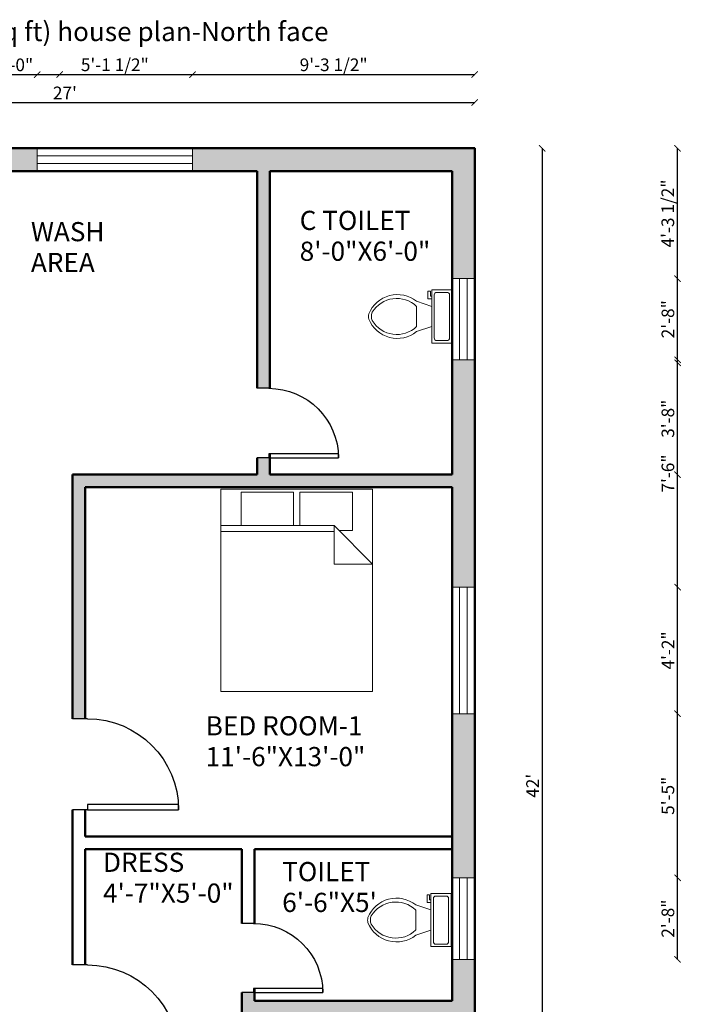
# Model space of a CAD drawing. Units: inches. Extents: x 1799 to 2247, y 1296 to 1881.
# Tile 4 of 4: x 1983 to 2247, y 1492 to 1881. Entities that reach past the tile are written whole.
import ezdxf

# ---------------------------------------------------------------- set-up
doc = ezdxf.new("R2010")
doc.units = ezdxf.units.IN
for name, color, linetype, lineweight in [('A-ANNO-DIMS', 2, 'Continuous', 18), ('A-ANNO-TEXT', 7, 'Continuous', 35), ('A-AREA-IDEN', 7, 'Continuous', 25), ('A-DOOR', 3, 'Continuous', 25), ('A-FLOR-FIXT', 9, 'Continuous', 18), ('A-FURN', 8, 'Continuous', 18), ('A-WALL', 7, 'Continuous', 50), ('window', 4, 'Continuous', 18)]:
    doc.layers.add(name, color=color, linetype=linetype, lineweight=lineweight)
doc.layers.add('A-WALL-PATT', color=18, linetype='Continuous', lineweight=13, true_color=0x000000)
doc.styles.get("Standard").update_dxf_attribs({"font": 'arial.ttf'})
doc.dimstyles.new('ISO-25', dxfattribs={"dimtxt": 5, "dimasz": 2.5, "dimexe": 1.25, "dimexo": 0.625, "dimtad": 1, "dimdec": 0, "dimlunit": 4, "dimtxsty": 'Standard', "dimblk": 'ARCHTICK', "dimcen": 2.5, "dimse1": 1, "dimse2": 1, "dimclrd": 1, "dimadec": 0, "dimazin": 0, "dimtfac": 1, "dimtdec": 0, "dimtmove": 0, "dimatfit": 3, "dimfxl": 1, "dimarcsym": 0})

# ---------------------------------------------------------------- blocks, each defined once
blk = doc.blocks.new('*U11')
for p, q in [((9.5, -6), (9.5, -2)), ((-10, -8.5), (-8, -8.5)), ((-10, -9.5), (-10, -8.5)), ((-7, -9.5), (-10, -9.5)), ((-8, -8.5), (-8, -8)), ((-7, -8), (-7, -9.5)), ((-4, -8), (-6, -14)), ((4, -8), (6, -14)), ((4, -14), (-4, -14))]:
    blk.add_line(p, q)
blk.add_lwpolyline([(10.5, -8), (10.5, 0), (-10.5, 0), (-10.5, -8)], close=True)
for points in [[(-9.5, -2), (-9.5, -6)], [(8.5, -1), (-8.5, -1)], [(-8.5, -7), (8.5, -7)]]:
    blk.add_lwpolyline(points)
for centre, radius, start, end in [((-8.62, -1.88), 0.884, 81.8699, 188.1301), ((8.62, -1.88), 0.884, 351.8699, 98.1301), ((-8.62, -6.12), 0.884, 171.8699, 278.1301), ((8.62, -6.12), 0.884, 261.8699, 8.1301), ((3.52, -21.58), 12.17, 141.4691, 247.9714), ((4.2, -21.82), 11.33, 136.3677, 238.9468), ((-3.52, -21.58), 12.17, 292.0284, 38.5307), ((-4.2, -21.82), 11.33, 301.053, 43.6321), ((0, -27.88), 4, 245.7318, 294.2682), ((0, -29), 4, 254.8605, 285.1395)]:
    blk.add_arc(centre, radius, start, end)
blk = doc.blocks.new('Bed - Queen')
for p, q in [((0, -80.00003), (0, 0)), ((0, 0), (59.99999, 0)), ((59.99999, 0), (59.99999, -80.00003)), ((7.99999, -1.2), (28.79998, -1.2)), ((7.99999, -14.4), (7.99999, -1.2)), ((28.79998, -1.2), (28.79998, -14.4)), ((31.19999, -1.2), (51.99999, -1.2)), ((31.19999, -14.4), (31.19999, -1.2)), ((51.99999, -1.2), (51.99999, -16.4)), ((0, -14.4), (44.8, -14.4)), ((59.99999, -29.6), (44.8, -14.4)), ((44.8, -14.4), (44.8, -29.6)), ((44.8, -16.8), (0, -16.8)), ((51.99999, -16.4), (46.79936, -16.4)), ((44.8, -29.6), (59.99999, -29.6)), ((59.99999, -80.00003), (0, -80.00003))]:
    blk.add_line(p, q)
blk = doc.blocks.new('*U12')
for p, q in [((0, 0), (0, -5)), ((30, 0), (30, -5))]:
    blk.add_line(p, q)
blk.add_lwpolyline([(0, 0), (0, 30), (1.75, 30), (1.75, 0)], close=True)
blk.add_arc((0, 0), 30, 0, 90)
blk = doc.blocks.new('_ArchTick')
at = {"color": 0, "linetype": 'ByBlock', "const_width": 0.15}
blk.add_lwpolyline([(-0.5, -0.5), (0.5, 0.5)], dxfattribs=at)
blk = doc.blocks.new('*D13')
at = {"layer": 'A-ANNO-DIMS', "color": 0, "lineweight": -2, "transparency": 16777216}
blk.add_line((1838.46, 1848.42), (2162.46, 1848.42), dxfattribs=at)
at = {"layer": 'Defpoints', "color": 0, "transparency": 16777216}
for p in [(2162.46, 1848.42), (1838.46, 1830.32), (2162.46, 1830.32)]:
    blk.add_point(p, dxfattribs=at)
at = {"layer": 'A-ANNO-DIMS', "color": 0, "lineweight": -2, "transparency": 16777216, "xscale": 2.5, "yscale": 2.5, "zscale": 2.5, "rotation": 180}
blk.add_blockref('_ArchTick', (1838.46, 1848.42), dxfattribs=at)
at = {"layer": 'A-ANNO-DIMS', "color": 0, "lineweight": -2, "transparency": 16777216, "xscale": 2.5, "yscale": 2.5, "zscale": 2.5}
blk.add_blockref('_ArchTick', (2162.46, 1848.42), dxfattribs=at)
at = {"layer": 'A-ANNO-DIMS', "color": 0, "transparency": 16777216, "insert": (2000.46, 1851.56), "char_height": 5, "attachment_point": 5}
blk.add_mtext("27'", dxfattribs=at)
blk = doc.blocks.new('*D14')
at = {"layer": 'A-ANNO-DIMS', "color": 0, "lineweight": -2, "transparency": 16777216}
blk.add_line((2189.08, 1830.32), (2189.08, 1326.32), dxfattribs=at)
at = {"layer": 'Defpoints', "color": 0, "transparency": 16777216}
for p in [(2162.46, 1830.32), (2162.46, 1326.32), (2189.08, 1326.32)]:
    blk.add_point(p, dxfattribs=at)
at = {"layer": 'A-ANNO-DIMS', "color": 0, "lineweight": -2, "transparency": 16777216, "xscale": 2.5, "yscale": 2.5, "zscale": 2.5}
for p, rotation in [((2189.08, 1830.32), 90), ((2189.08, 1326.32), 270)]:
    blk.add_blockref('_ArchTick', p, dxfattribs=dict(at, rotation=rotation))
at = {"layer": 'A-ANNO-DIMS', "color": 0, "transparency": 16777216, "insert": (2185.95, 1578.32), "char_height": 5, "attachment_point": 5, "rotation": 90}
blk.add_mtext("42'", dxfattribs=at)
blk = doc.blocks.new('*D35')
at = {"layer": 'A-ANNO-DIMS', "color": 1, "lineweight": -2, "transparency": 16777216}
blk.add_line((1960.46, 1297.17), (2076.46, 1297.17), dxfattribs=at)
at = {"layer": 'Defpoints', "color": 0, "transparency": 16777216}
for p in [(1960.46, 1821.32), (2076.46, 1821.32), (2076.46, 1297.17)]:
    blk.add_point(p, dxfattribs=at)
at = {"layer": 'A-ANNO-DIMS', "color": 1, "lineweight": -2, "transparency": 16777216, "xscale": 2.5, "yscale": 2.5, "zscale": 2.5, "rotation": 180}
blk.add_blockref('_ArchTick', (1960.46, 1297.17), dxfattribs=at)
at = {"layer": 'A-ANNO-DIMS', "color": 1, "lineweight": -2, "transparency": 16777216, "xscale": 2.5, "yscale": 2.5, "zscale": 2.5}
blk.add_blockref('_ArchTick', (2076.46, 1297.17), dxfattribs=at)
at = {"layer": 'A-ANNO-DIMS', "color": 0, "transparency": 16777216, "insert": (2018.46, 1300.35), "char_height": 5, "attachment_point": 5}
blk.add_mtext('9\'-8"', dxfattribs=at)
blk = doc.blocks.new('*D39')
at = {"layer": 'A-ANNO-DIMS', "color": 1, "lineweight": -2, "transparency": 16777216}
blk.add_line((2242.61, 1509.73), (2242.61, 1541.93), dxfattribs=at)
at = {"layer": 'Defpoints', "color": 0, "transparency": 16777216}
for p in [(2162.46, 1541.93), (2242.61, 1541.93), (2162.46, 1509.73)]:
    blk.add_point(p, dxfattribs=at)
at = {"layer": 'A-ANNO-DIMS', "color": 1, "lineweight": -2, "transparency": 16777216, "xscale": 2.5, "yscale": 2.5, "zscale": 2.5}
for p, rotation in [((2242.61, 1541.93), 90), ((2242.61, 1509.73), 270)]:
    blk.add_blockref('_ArchTick', p, dxfattribs=dict(at, rotation=rotation))
at = {"layer": 'A-ANNO-DIMS', "color": 0, "transparency": 16777216, "insert": (2239.43, 1525.83), "char_height": 5, "attachment_point": 5, "rotation": 90}
blk.add_mtext('2\'-8"', dxfattribs=at)
blk = doc.blocks.new('*D40')
at = {"layer": 'A-ANNO-DIMS', "color": 1, "lineweight": -2, "transparency": 16777216}
blk.add_line((2242.61, 1541.93), (2242.61, 1606.83), dxfattribs=at)
at = {"layer": 'Defpoints', "color": 0, "transparency": 16777216}
for p in [(2162.46, 1606.83), (2242.61, 1606.83), (2162.46, 1541.93)]:
    blk.add_point(p, dxfattribs=at)
at = {"layer": 'A-ANNO-DIMS', "color": 1, "lineweight": -2, "transparency": 16777216, "xscale": 2.5, "yscale": 2.5, "zscale": 2.5}
for p, rotation in [((2242.61, 1606.83), 90), ((2242.61, 1541.93), 270)]:
    blk.add_blockref('_ArchTick', p, dxfattribs=dict(at, rotation=rotation))
at = {"layer": 'A-ANNO-DIMS', "color": 0, "transparency": 16777216, "insert": (2239.44, 1574.38), "char_height": 5, "attachment_point": 5, "rotation": 90}
blk.add_mtext('5\'-5"', dxfattribs=at)
blk = doc.blocks.new('*D41')
at = {"layer": 'A-ANNO-DIMS', "color": 1, "lineweight": -2, "transparency": 16777216}
blk.add_line((2242.61, 1606.83), (2242.61, 1656.83), dxfattribs=at)
at = {"layer": 'Defpoints', "color": 0, "transparency": 16777216}
for p in [(2162.46, 1656.83), (2242.61, 1656.83), (2162.46, 1606.83)]:
    blk.add_point(p, dxfattribs=at)
at = {"layer": 'A-ANNO-DIMS', "color": 1, "lineweight": -2, "transparency": 16777216, "xscale": 2.5, "yscale": 2.5, "zscale": 2.5}
for p, rotation in [((2242.61, 1656.83), 90), ((2242.61, 1606.83), 270)]:
    blk.add_blockref('_ArchTick', p, dxfattribs=dict(at, rotation=rotation))
at = {"layer": 'A-ANNO-DIMS', "color": 0, "transparency": 16777216, "insert": (2239.47, 1631.83), "char_height": 5, "attachment_point": 5, "rotation": 90}
blk.add_mtext('4\'-2"', dxfattribs=at)
blk = doc.blocks.new('*D42')
at = {"layer": 'A-ANNO-DIMS', "color": 1, "lineweight": -2, "transparency": 16777216}
blk.add_line((2242.61, 1656.83), (2242.61, 1746.71), dxfattribs=at)
at = {"layer": 'Defpoints', "color": 0, "transparency": 16777216}
for p in [(2162.46, 1746.71), (2242.61, 1746.71), (2162.46, 1656.83)]:
    blk.add_point(p, dxfattribs=at)
at = {"layer": 'A-ANNO-DIMS', "color": 1, "lineweight": -2, "transparency": 16777216, "xscale": 2.5, "yscale": 2.5, "zscale": 2.5}
for p, rotation in [((2242.61, 1746.71), 90), ((2242.61, 1656.83), 270)]:
    blk.add_blockref('_ArchTick', p, dxfattribs=dict(at, rotation=rotation))
at = {"layer": 'A-ANNO-DIMS', "color": 0, "transparency": 16777216, "insert": (2239.43, 1701.77), "char_height": 5, "attachment_point": 5, "rotation": 90}
blk.add_mtext('7\'-6"', dxfattribs=at)
blk = doc.blocks.new('*D43')
at = {"layer": 'A-ANNO-DIMS', "color": 1, "lineweight": -2, "transparency": 16777216}
blk.add_line((2242.61, 1746.71), (2242.61, 1778.8), dxfattribs=at)
at = {"layer": 'Defpoints', "color": 0, "transparency": 16777216}
for p in [(2162.46, 1778.8), (2242.61, 1778.8), (2162.46, 1746.71)]:
    blk.add_point(p, dxfattribs=at)
at = {"layer": 'A-ANNO-DIMS', "color": 1, "lineweight": -2, "transparency": 16777216, "xscale": 2.5, "yscale": 2.5, "zscale": 2.5}
for p, rotation in [((2242.61, 1778.8), 90), ((2242.61, 1746.71), 270)]:
    blk.add_blockref('_ArchTick', p, dxfattribs=dict(at, rotation=rotation))
at = {"layer": 'A-ANNO-DIMS', "color": 0, "transparency": 16777216, "insert": (2239.43, 1762.75), "char_height": 5, "attachment_point": 5, "rotation": 90}
blk.add_mtext('2\'-8"', dxfattribs=at)
blk = doc.blocks.new('*D44')
at = {"layer": 'A-ANNO-DIMS', "color": 1, "lineweight": -2, "transparency": 16777216}
blk.add_line((2242.61, 1778.8), (2242.61, 1830.32), dxfattribs=at)
at = {"layer": 'Defpoints', "color": 0, "transparency": 16777216}
for p in [(2162.46, 1830.32), (2242.61, 1830.32), (2162.46, 1778.8)]:
    blk.add_point(p, dxfattribs=at)
at = {"layer": 'A-ANNO-DIMS', "color": 1, "lineweight": -2, "transparency": 16777216, "xscale": 2.5, "yscale": 2.5, "zscale": 2.5}
for p, rotation in [((2242.61, 1830.32), 90), ((2242.61, 1778.8), 270)]:
    blk.add_blockref('_ArchTick', p, dxfattribs=dict(at, rotation=rotation))
at = {"layer": 'A-ANNO-DIMS', "color": 0, "transparency": 16777216, "insert": (2239.39, 1804.56), "char_height": 5, "attachment_point": 5, "rotation": 90}
blk.add_mtext('4\'-3 1/2"', dxfattribs=at)
blk = doc.blocks.new('*D48')
at = {"layer": 'A-ANNO-DIMS', "color": 1, "lineweight": -2, "transparency": 16777216}
blk.add_line((1962.42, 1859.47), (1998.36, 1859.47), dxfattribs=at)
at = {"layer": 'Defpoints', "color": 0, "transparency": 16777216}
for p in [(1998.36, 1859.47), (1962.42, 1353.51), (1998.36, 1353.51)]:
    blk.add_point(p, dxfattribs=at)
at = {"layer": 'A-ANNO-DIMS', "color": 1, "lineweight": -2, "transparency": 16777216, "xscale": 2.5, "yscale": 2.5, "zscale": 2.5, "rotation": 180}
blk.add_blockref('_ArchTick', (1962.42, 1859.47), dxfattribs=at)
at = {"layer": 'A-ANNO-DIMS', "color": 1, "lineweight": -2, "transparency": 16777216, "xscale": 2.5, "yscale": 2.5, "zscale": 2.5}
blk.add_blockref('_ArchTick', (1998.36, 1859.47), dxfattribs=at)
at = {"layer": 'A-ANNO-DIMS', "color": 0, "transparency": 16777216, "insert": (1980.39, 1862.65), "char_height": 5, "attachment_point": 5}
blk.add_mtext('3\'-0"', dxfattribs=at)
blk = doc.blocks.new('*D53')
at = {"layer": 'A-ANNO-DIMS', "color": 1, "lineweight": -2, "transparency": 16777216}
blk.add_line((1989.49, 1859.47), (2050.89, 1859.47), dxfattribs=at)
at = {"layer": 'Defpoints', "color": 0, "transparency": 16777216}
for p in [(2050.89, 1859.47), (1989.49, 1830.32), (2050.89, 1830.32)]:
    blk.add_point(p, dxfattribs=at)
at = {"layer": 'A-ANNO-DIMS', "color": 1, "lineweight": -2, "transparency": 16777216, "xscale": 2.5, "yscale": 2.5, "zscale": 2.5, "rotation": 180}
blk.add_blockref('_ArchTick', (1989.49, 1859.47), dxfattribs=at)
at = {"layer": 'A-ANNO-DIMS', "color": 1, "lineweight": -2, "transparency": 16777216, "xscale": 2.5, "yscale": 2.5, "zscale": 2.5}
blk.add_blockref('_ArchTick', (2050.89, 1859.47), dxfattribs=at)
at = {"layer": 'A-ANNO-DIMS', "color": 0, "transparency": 16777216, "insert": (2020.19, 1862.68), "char_height": 5, "attachment_point": 5}
blk.add_mtext('5\'-1 1/2"', dxfattribs=at)
blk = doc.blocks.new('*D54')
at = {"layer": 'A-ANNO-DIMS', "color": 1, "lineweight": -2, "transparency": 16777216}
blk.add_line((2050.89, 1859.47), (2162.46, 1859.47), dxfattribs=at)
at = {"layer": 'Defpoints', "color": 0, "transparency": 16777216}
for p in [(2162.46, 1859.47), (2050.89, 1830.32), (2162.46, 1830.32)]:
    blk.add_point(p, dxfattribs=at)
at = {"layer": 'A-ANNO-DIMS', "color": 1, "lineweight": -2, "transparency": 16777216, "xscale": 2.5, "yscale": 2.5, "zscale": 2.5, "rotation": 180}
blk.add_blockref('_ArchTick', (2050.89, 1859.47), dxfattribs=at)
at = {"layer": 'A-ANNO-DIMS', "color": 1, "lineweight": -2, "transparency": 16777216, "xscale": 2.5, "yscale": 2.5, "zscale": 2.5}
blk.add_blockref('_ArchTick', (2162.46, 1859.47), dxfattribs=at)
at = {"layer": 'A-ANNO-DIMS', "color": 0, "transparency": 16777216, "insert": (2106.68, 1862.68), "char_height": 5, "attachment_point": 5}
blk.add_mtext('9\'-3 1/2"', dxfattribs=at)
blk = doc.blocks.new('*D55')
at = {"layer": 'A-ANNO-DIMS', "color": 1, "lineweight": -2, "transparency": 16777216}
blk.add_line((2242.61, 1701.32), (2242.61, 1745.53), dxfattribs=at)
at = {"layer": 'Defpoints', "color": 0, "transparency": 16777216}
for p in [(1847.46, 1745.53), (2242.61, 1745.53), (1847.46, 1701.32)]:
    blk.add_point(p, dxfattribs=at)
at = {"layer": 'A-ANNO-DIMS', "color": 1, "lineweight": -2, "transparency": 16777216, "xscale": 2.5, "yscale": 2.5, "zscale": 2.5}
for p, rotation in [((2242.61, 1745.53), 90), ((2242.61, 1701.32), 270)]:
    blk.add_blockref('_ArchTick', p, dxfattribs=dict(at, rotation=rotation))
at = {"layer": 'A-ANNO-DIMS', "color": 0, "transparency": 16777216, "insert": (2239.43, 1723.42), "char_height": 5, "attachment_point": 5, "rotation": 90}
blk.add_mtext('3\'-8"', dxfattribs=at)
blk = doc.blocks.new('*D58')
at = {"layer": 'A-ANNO-DIMS', "color": 1, "lineweight": -2, "transparency": 16777216}
blk.add_line((1809.31, 1568.87), (1809.31, 1604.81), dxfattribs=at)
at = {"layer": 'Defpoints', "color": 0, "transparency": 16777216}
for p in [(1809.31, 1604.81), (2003.46, 1604.81), (2003.46, 1568.87)]:
    blk.add_point(p, dxfattribs=at)
at = {"layer": 'A-ANNO-DIMS', "color": 1, "lineweight": -2, "transparency": 16777216, "xscale": 2.5, "yscale": 2.5, "zscale": 2.5}
for p, rotation in [((1809.31, 1604.81), 90), ((1809.31, 1568.87), 270)]:
    blk.add_blockref('_ArchTick', p, dxfattribs=dict(at, rotation=rotation))
at = {"layer": 'A-ANNO-DIMS', "color": 0, "transparency": 16777216, "insert": (1806.13, 1586.84), "char_height": 5, "attachment_point": 5, "rotation": 90}
blk.add_mtext('3\'-0"', dxfattribs=at)
blk = doc.blocks.new('*D59')
at = {"layer": 'A-ANNO-DIMS', "color": 1, "lineweight": -2, "transparency": 16777216}
blk.add_line((1809.31, 1507.52), (1809.31, 1568.87), dxfattribs=at)
at = {"layer": 'Defpoints', "color": 0, "transparency": 16777216}
for p in [(1809.31, 1568.87), (2003.46, 1568.87), (2003.46, 1507.52)]:
    blk.add_point(p, dxfattribs=at)
at = {"layer": 'A-ANNO-DIMS', "color": 1, "lineweight": -2, "transparency": 16777216, "xscale": 2.5, "yscale": 2.5, "zscale": 2.5}
for p, rotation in [((1809.31, 1568.87), 90), ((1809.31, 1507.52), 270)]:
    blk.add_blockref('_ArchTick', p, dxfattribs=dict(at, rotation=rotation))
at = {"layer": 'A-ANNO-DIMS', "color": 0, "transparency": 16777216, "insert": (1806.1, 1538.19), "char_height": 5, "attachment_point": 5, "rotation": 90}
blk.add_mtext('5\'-1 1/2"', dxfattribs=at)
blk = doc.blocks.new('*D60')
at = {"layer": 'A-ANNO-DIMS', "color": 1, "lineweight": -2, "transparency": 16777216}
blk.add_line((1809.31, 1471.58), (1809.31, 1507.52), dxfattribs=at)
at = {"layer": 'Defpoints', "color": 0, "transparency": 16777216}
for p in [(1809.31, 1507.52), (2003.46, 1507.52), (2003.46, 1471.58)]:
    blk.add_point(p, dxfattribs=at)
at = {"layer": 'A-ANNO-DIMS', "color": 1, "lineweight": -2, "transparency": 16777216, "xscale": 2.5, "yscale": 2.5, "zscale": 2.5}
for p, rotation in [((1809.31, 1507.52), 90), ((1809.31, 1471.58), 270)]:
    blk.add_blockref('_ArchTick', p, dxfattribs=dict(at, rotation=rotation))
at = {"layer": 'A-ANNO-DIMS', "color": 0, "transparency": 16777216, "insert": (1806.13, 1489.55), "char_height": 5, "attachment_point": 5, "rotation": 90}
blk.add_mtext('3\'-0"', dxfattribs=at)
blk = doc.blocks.new('*D64')
at = {"layer": 'A-ANNO-DIMS', "color": 1, "lineweight": -2, "transparency": 16777216}
blk.add_line((1809.31, 1496.56), (1809.31, 1523.93), dxfattribs=at)
at = {"layer": 'Defpoints', "color": 0, "transparency": 16777216}
for p in [(1809.31, 1523.93), (2070.46, 1523.93), (2070.46, 1496.56)]:
    blk.add_point(p, dxfattribs=at)
at = {"layer": 'A-ANNO-DIMS', "color": 1, "lineweight": -2, "transparency": 16777216, "xscale": 2.5, "yscale": 2.5, "zscale": 2.5}
for p, rotation in [((1809.31, 1523.93), 90), ((1809.31, 1496.56), 270)]:
    blk.add_blockref('_ArchTick', p, dxfattribs=dict(at, rotation=rotation))
at = {"layer": 'A-ANNO-DIMS', "color": 0, "transparency": 16777216, "insert": (1806.09, 1510.25), "char_height": 5, "attachment_point": 5, "rotation": 90}
blk.add_mtext('2\'-3 1/2"', dxfattribs=at)
blk = doc.blocks.new('*D65')
at = {"layer": 'A-ANNO-DIMS', "color": 1, "lineweight": -2, "transparency": 16777216}
blk.add_line((1809.31, 1523.93), (1809.31, 1553.32), dxfattribs=at)
at = {"layer": 'Defpoints', "color": 0, "transparency": 16777216}
for p in [(1809.31, 1553.32), (2070.46, 1553.32), (2070.46, 1523.93)]:
    blk.add_point(p, dxfattribs=at)
at = {"layer": 'A-ANNO-DIMS', "color": 1, "lineweight": -2, "transparency": 16777216, "xscale": 2.5, "yscale": 2.5, "zscale": 2.5}
for p, rotation in [((1809.31, 1553.32), 90), ((1809.31, 1523.93), 270)]:
    blk.add_blockref('_ArchTick', p, dxfattribs=dict(at, rotation=rotation))
at = {"layer": 'A-ANNO-DIMS', "color": 0, "transparency": 16777216, "insert": (1806.1, 1538.62), "char_height": 5, "attachment_point": 5, "rotation": 90}
blk.add_mtext('2\'-5 1/2"', dxfattribs=at)
blk = doc.blocks.new('*D66')
at = {"layer": 'A-ANNO-DIMS', "color": 1, "lineweight": -2, "transparency": 16777216}
blk.add_line((2120.1, 1297.17), (2153.1, 1297.17), dxfattribs=at)
at = {"layer": 'Defpoints', "color": 0, "transparency": 16777216}
for p in [(2120.1, 1525.25), (2153.1, 1514.75), (2153.1, 1297.17)]:
    blk.add_point(p, dxfattribs=at)
at = {"layer": 'A-ANNO-DIMS', "color": 1, "lineweight": -2, "transparency": 16777216, "xscale": 2.5, "yscale": 2.5, "zscale": 2.5, "rotation": 180}
blk.add_blockref('_ArchTick', (2120.1, 1297.17), dxfattribs=at)
at = {"layer": 'A-ANNO-DIMS', "color": 1, "lineweight": -2, "transparency": 16777216, "xscale": 2.5, "yscale": 2.5, "zscale": 2.5}
blk.add_blockref('_ArchTick', (2153.1, 1297.17), dxfattribs=at)
at = {"layer": 'A-ANNO-DIMS', "color": 0, "transparency": 16777216, "insert": (2136.6, 1300.35), "char_height": 5, "attachment_point": 5}
blk.add_mtext('2\'-9"', dxfattribs=at)
blk = doc.blocks.new('*D67')
at = {"layer": 'A-ANNO-DIMS', "color": 1, "lineweight": -2, "transparency": 16777216}
blk.add_line((1809.31, 1514.75), (1809.31, 1535.75), dxfattribs=at)
at = {"layer": 'Defpoints', "color": 0, "transparency": 16777216}
for p in [(1809.31, 1535.75), (2145.1, 1535.75), (2145.1, 1514.75)]:
    blk.add_point(p, dxfattribs=at)
at = {"layer": 'A-ANNO-DIMS', "color": 1, "lineweight": -2, "transparency": 16777216, "xscale": 2.5, "yscale": 2.5, "zscale": 2.5}
for p, rotation in [((1809.31, 1535.75), 90), ((1809.31, 1514.75), 270)]:
    blk.add_blockref('_ArchTick', p, dxfattribs=dict(at, rotation=rotation))
at = {"layer": 'A-ANNO-DIMS', "color": 0, "transparency": 16777216, "insert": (1806.13, 1525.25), "char_height": 5, "attachment_point": 5, "rotation": 90}
blk.add_mtext('1\'-9"', dxfattribs=at)
blk = doc.blocks.new('*D68')
at = {"layer": 'A-ANNO-DIMS', "color": 1, "lineweight": -2, "transparency": 16777216}
for p, q in [((1809.31, 1553.32), (1809.31, 1581.54)), ((1809.31, 1535.75), (1809.31, 1553.32))]:
    blk.add_line(p, q, dxfattribs=at)
at = {"layer": 'Defpoints', "color": 0, "transparency": 16777216}
for p in [(1809.31, 1553.32), (2153.46, 1553.32), (2153.1, 1535.75)]:
    blk.add_point(p, dxfattribs=at)
at = {"layer": 'A-ANNO-DIMS', "color": 1, "lineweight": -2, "transparency": 16777216, "xscale": 2.5, "yscale": 2.5, "zscale": 2.5}
for p, rotation in [((1809.31, 1553.32), 90), ((1809.31, 1535.75), 270)]:
    blk.add_blockref('_ArchTick', p, dxfattribs=dict(at, rotation=rotation))
at = {"layer": 'A-ANNO-DIMS', "color": 0, "transparency": 16777216, "insert": (1806.1, 1568.68), "char_height": 5, "attachment_point": 5, "rotation": 90}
blk.add_mtext('1\'-5 1/2"', dxfattribs=at)

msp = doc.modelspace()

# ---------------------------------------------------------------- hatches: boundary and pattern name
at = {"layer": 'A-WALL-PATT'}
h = msp.add_hatch(color=256, dxfattribs=at)
h.dxf.hatch_style = 1
h.paths.add_polyline_path([(1847.46, 1821.32), (1883.11, 1821.32), (1883.11, 1830.32), (1838.46, 1830.32), (1838.46, 1618.8), (1847.46, 1618.8)])
h.paths.add_polyline_path([(1847.46, 1534.31), (1838.46, 1534.31), (1838.46, 1444.97), (1847.46, 1444.97)])
h.paths.add_polyline_path([(1847.46, 1404.13), (1838.46, 1404.13), (1838.46, 1353.51), (1847.46, 1353.51), (1962.42, 1353.51), (1962.42, 1359.5, -0.020971), (1962.55, 1362.51), (1847.46, 1362.51)])
h.paths.add_polyline_path([(2162.46, 1509.73), (2153.46, 1509.73), (2153.46, 1493.32), (2075.46, 1493.32), (2075.46, 1496.56), (2075.02, 1496.56), (2070.46, 1496.56), (2070.46, 1488.32), (2153.46, 1488.32), (2153.46, 1335.32), (2119.37, 1335.32), (2119.37, 1326.32), (2162.46, 1326.32)])
h.paths.add_polyline_path([(2059.58, 1335.32), (2008.46, 1335.32), (2008.46, 1353.51), (2003.46, 1353.51), (2003.46, 1335.32), (2003.46, 1326.32), (2059.58, 1326.32)])
h.paths.add_polyline_path([(2008.46, 1471.58), (2003.46, 1471.58), (2003.46, 1460.32), (1847.46, 1460.32), (1847.46, 1455.32), (2003.46, 1455.32), (2003.46, 1362.51), (2008.46, 1362.51)])
h.paths.add_polyline_path([(2008.46, 1362.51), (2003.46, 1362.51), (2003.46, 1353.51), (2008.46, 1353.51)])
h.paths.add_polyline_path([(2003.46, 1362.51), (1998.36, 1362.51), (1998.36, 1359.5), (1998.36, 1353.51), (2003.46, 1353.51)])
h.paths.add_polyline_path([(1989.49, 1830.32), (1953.2, 1830.32), (1953.2, 1821.32), (1955.46, 1821.32), (1955.46, 1701.32), (1950.83, 1701.32), (1950.83, 1696.32), (1960.46, 1696.32), (1960.46, 1821.32), (1989.49, 1821.32)])
h.paths.add_polyline_path([(2162.46, 1606.83), (2153.46, 1606.83), (2153.46, 1541.93), (2162.46, 1541.93)])
h.paths.add_polyline_path([(2162.46, 1746.71), (2153.46, 1746.71), (2153.46, 1701.32), (2081.46, 1701.32), (2081.46, 1707.91), (2081.05, 1707.91), (2076.46, 1707.91), (2076.46, 1701.32), (2003.46, 1701.32), (2003.46, 1604.81), (2008.46, 1604.81), (2008.46, 1696.32), (2153.46, 1696.32), (2153.46, 1656.83), (2162.46, 1656.83)])
h.paths.add_polyline_path([(2162.46, 1830.32), (2050.89, 1830.32), (2050.89, 1821.32), (2076.46, 1821.32), (2076.46, 1735.44), (2081.05, 1735.44, -0.003736), (2081.46, 1735.44), (2081.46, 1821.32), (2153.46, 1821.32), (2153.46, 1778.8), (2162.46, 1778.8)])
h.paths.add_polyline_path([(1961.29, 1344.27), (2000.99, 1344.27), (2000.99, 1355.65), (1961.29, 1355.65)], flags=9)
h.paths.add_polyline_path([(1882.83, 1491.06), (1947.74, 1491.06), (1947.74, 1502.69), (1882.83, 1502.69)], flags=9)
h.paths.add_polyline_path([(1882.8, 1503.23), (1950.9, 1503.23), (1950.9, 1514.99), (1882.8, 1514.99)], flags=9)
h.paths.add_polyline_path([(2045.91, 1444.14), (2110.82, 1444.14), (2110.82, 1455.75), (2045.91, 1455.75)], flags=9)
h.paths.add_polyline_path([(2045.88, 1456.29), (2116.91, 1456.29), (2116.91, 1468.06), (2045.88, 1468.06)], flags=9)
h.paths.add_polyline_path([(2084.43, 1526.38), (2124.38, 1526.38), (2124.38, 1537.99), (2084.43, 1537.99)], flags=9)
h.paths.add_polyline_path([(2084.4, 1538.53), (2125.41, 1538.53), (2125.41, 1550.3), (2084.4, 1550.3)], flags=9)
h.paths.add_polyline_path([(2013.59, 1530.05), (2066.72, 1530.05), (2066.72, 1541.67), (2013.59, 1541.67)], flags=9)
h.paths.add_polyline_path([(2013.56, 1542.21), (2053.98, 1542.21), (2053.98, 1553.97), (2013.56, 1553.97)], flags=9)
h.paths.add_polyline_path([(2054.17, 1583.99), (2119.08, 1583.99), (2119.08, 1595.62), (2054.17, 1595.62)], flags=9)
h.paths.add_polyline_path([(2054.14, 1596.16), (2125.17, 1596.16), (2125.17, 1607.93), (2054.14, 1607.93)], flags=9)
h.paths.add_polyline_path([(2091.32, 1783.78), (2144.45, 1783.78), (2144.45, 1795.39), (2091.32, 1795.39)], flags=25)
h.paths.add_polyline_path([(2091.3, 1795.93), (2142.9, 1795.93), (2142.9, 1807.7), (2091.3, 1807.7)], flags=25)
h.paths.add_polyline_path([(1985.13, 1779.5), (2017.8, 1779.5), (2017.8, 1790.88), (1985.13, 1790.88)], flags=9)
h.paths.add_polyline_path([(1985.08, 1791.49), (2020.79, 1791.49), (2020.79, 1803.25), (1985.08, 1803.25)], flags=9)
h.paths.add_polyline_path([(1879.15, 1761.55), (1938.17, 1761.55), (1938.17, 1773.17), (1879.15, 1773.17)], flags=9)
h.paths.add_polyline_path([(1879.13, 1773.71), (1929.55, 1773.71), (1929.55, 1785.47), (1879.13, 1785.47)], flags=9)

# ---------------------------------------------------------------- linework, layer by layer
at = {"layer": 'A-WALL'}
for p, q in [((1960.46, 1821.32), (2076.46, 1821.32)), ((2076.46, 1821.32), (2076.46, 1735.44)), ((2081.46, 1821.32), (2081.46, 1735.44)), ((2081.46, 1821.32), (2153.46, 1821.32)), ((2153.46, 1821.32), (2153.46, 1701.32)), ((2081.46, 1709.51), (2081.46, 1701.32)), ((2076.46, 1707.91), (2076.46, 1701.32)), ((2003.46, 1701.32), (2076.46, 1701.32)), ((2003.46, 1604.81), (2003.46, 1701.32)), ((2081.46, 1701.32), (2153.46, 1701.32)), ((2008.46, 1696.32), (2153.46, 1696.32)), ((2008.46, 1604.81), (2008.46, 1696.32)), ((2153.46, 1696.32), (2153.46, 1493.32)), ((2003.46, 1507.52), (2003.46, 1568.87)), ((2008.46, 1558.32), (2008.46, 1568.87)), ((2008.46, 1558.32), (2153.46, 1558.32)), ((2008.46, 1553.32), (2070.46, 1553.32)), ((2008.46, 1507.52), (2008.46, 1553.32)), ((2070.46, 1553.32), (2070.46, 1523.93)), ((2075.46, 1553.32), (2075.46, 1523.93)), ((2075.46, 1553.32), (2153.46, 1553.32)), ((2070.46, 1496.56), (2070.46, 1488.32)), ((2075.46, 1498.16), (2075.46, 1493.32)), ((2075.46, 1493.32), (2153.46, 1493.32))]:
    msp.add_line(p, q, dxfattribs=at)
msp.add_lwpolyline([(1838.46, 1353.51), (1838.46, 1830.32), (2162.46, 1830.32), (2162.46, 1326.32), (2003.46, 1326.32)], dxfattribs=at)
at = {"layer": 'window'}
for p, q in [((2050.89, 1830.32), (1989.49, 1830.32)), ((1989.49, 1830.32), (1989.49, 1821.32)), ((2050.89, 1821.32), (2050.89, 1830.32)), ((2050.89, 1827.32), (1989.49, 1827.32)), ((2050.89, 1824.32), (1989.49, 1824.32)), ((1989.49, 1821.32), (2050.89, 1821.32)), ((2162.46, 1778.8), (2153.46, 1778.8)), ((2153.46, 1778.8), (2153.46, 1746.71)), ((2156.46, 1746.71), (2156.46, 1778.8)), ((2159.46, 1746.71), (2159.46, 1778.8)), ((2162.46, 1746.71), (2162.46, 1778.8)), ((2153.46, 1746.71), (2162.46, 1746.71)), ((2162.46, 1656.83), (2153.46, 1656.83)), ((2153.46, 1656.83), (2153.46, 1606.83)), ((2156.46, 1606.83), (2156.46, 1656.83)), ((2159.46, 1606.83), (2159.46, 1656.83)), ((2162.46, 1606.83), (2162.46, 1656.83)), ((2153.46, 1606.83), (2162.46, 1606.83)), ((2162.46, 1541.93), (2153.46, 1541.93)), ((2153.46, 1541.93), (2153.46, 1509.73)), ((2156.46, 1509.73), (2156.46, 1541.93)), ((2159.46, 1509.73), (2159.46, 1541.93)), ((2162.46, 1509.73), (2162.46, 1541.93)), ((2153.46, 1509.73), (2162.46, 1509.73))]:
    msp.add_line(p, q, dxfattribs=at)

# ---------------------------------------------------------------- block references
at = {"layer": 'A-DOOR', "rotation": 270}
for p, xscale, yscale, zscale in [((2081.05, 1707.91), -0.9177236943581608, 0.9177236943581608, 0.9177236943581608), ((2009.45, 1568.87), -1.197883670562129, 1.197883670562129, 1.197883670562129), ((2075.02, 1496.56), -0.9122280791154926, 0.9122280791154926, 0.9122280791154926), ((2009.45, 1471.58), -1.197883670562129, 1.197883670562129, 1.197883670562129)]:
    msp.add_blockref('*U12', p, dxfattribs=dict(at, xscale=xscale, yscale=yscale, zscale=zscale))
at = {"layer": 'A-FLOR-FIXT', "rotation": 270}
for p in [(2153.46, 1763.84), (2153.1, 1525.25)]:
    msp.add_blockref('*U11', p, dxfattribs=at)
at = {"layer": 'A-FURN'}
msp.add_blockref('Bed - Queen', (2062.07, 1695.6), dxfattribs=at)

# ---------------------------------------------------------------- texts
at = {"layer": 'A-ANNO-TEXT'}
msp.add_text('27X42(1134 sq ft) house plan-North face', height=7.5834, dxfattribs=at).set_placement((1913.09, 1872.69))
at = {"layer": 'A-AREA-IDEN'}
for s, height, p in [('C TOILET', 7.583, (2093.26, 1798.03)), ('WASH', 7.583, (1987.04, 1793.58)), ('8\'-0"X6\'-0"', 7.5834, (2093.26, 1785.84)), ('AREA', 7.583, (1987.04, 1781.4)), ('BED ROOM-1', 7.583, (2056.1, 1598.25)), ('11\'-6"X13\'-0"', 7.5834, (2056.1, 1586.07)), ('DRESS', 7.583, (2015.52, 1544.3)), ('TOILET', 7.583, (2086.36, 1540.62)), ('4\'-7"X5\'-0"', 7.5834, (2015.52, 1532.12)), ('6\'-6"X5\'', 7.583, (2086.36, 1528.44))]:
    msp.add_text(s, height=height, dxfattribs=at).set_placement(p)

# ---------------------------------------------------------------- dimensions: what is measured, and where the dimension line sits
at = {"layer": 'A-ANNO-DIMS'}
for base, p1, p2, override, picture, middle in [((2050.89, 1859.47), (1989.49, 1830.32), (2050.89, 1830.32), {"dimdec": 1, "dimlfac": 1, "dimrnd": 0, "dimzin": 1, "dimdsep": 46, "dimlunit": 4, "dimfrac": 2}, '*D53', (2020.19, 1862.68)), ((2162.46, 1859.47), (2050.89, 1830.32), (2162.46, 1830.32), {"dimdec": 1, "dimlfac": 1, "dimrnd": 0, "dimzin": 1, "dimdsep": 46, "dimlunit": 4, "dimfrac": 2}, '*D54', (2106.68, 1862.68)), ((1998.36, 1859.47), (1962.42, 1353.51), (1998.36, 1353.51), {"dimdec": 1, "dimlfac": 1, "dimrnd": 0, "dimzin": 1, "dimdsep": 46, "dimlunit": 4, "dimfrac": 2}, '*D48', (1980.39, 1862.65)), ((2162.46, 1848.42), (1838.46, 1830.32), (2162.46, 1830.32), {"dimclrd": 0, "dimclre": 0, "dimclrt": 0}, '*D13', (2000.46, 1851.56)), ((2076.46, 1297.17), (1960.46, 1821.32), (2076.46, 1821.32), {"dimdec": 1, "dimlfac": 1, "dimrnd": 0, "dimzin": 1, "dimdsep": 46, "dimlunit": 4, "dimfrac": 2}, '*D35', (2018.46, 1300.35)), ((2153.1, 1297.17), (2120.1, 1525.25), (2153.1, 1514.75), {"dimdec": 1, "dimlfac": 1, "dimrnd": 0, "dimzin": 1, "dimdsep": 46, "dimlunit": 4, "dimfrac": 2}, '*D66', (2136.6, 1300.35))]:
    dim = msp.add_linear_dim(base=base, p1=p1, p2=p2, dimstyle='ISO-25', override=override, dxfattribs=at)
    dim.commit()
    dim.dimension.update_dxf_attribs({"geometry": picture, "text_midpoint": middle})
for base, p1, p2, override, picture, middle in [((2189.08, 1326.32), (2162.46, 1830.32), (2162.46, 1326.32), {"dimclrd": 0, "dimclre": 0, "dimclrt": 0}, '*D14', (2185.95, 1578.32)), ((2242.61, 1830.32), (2162.46, 1778.8), (2162.46, 1830.32), {"dimdec": 1, "dimlfac": 1, "dimrnd": 0, "dimzin": 1, "dimdsep": 46, "dimlunit": 4, "dimfrac": 2}, '*D44', (2239.39, 1804.56)), ((2242.61, 1778.8), (2162.46, 1746.71), (2162.46, 1778.8), {"dimdec": 1, "dimlfac": 1, "dimrnd": 0, "dimzin": 1, "dimdsep": 46, "dimlunit": 4, "dimfrac": 2}, '*D43', (2239.43, 1762.75)), ((2242.61, 1746.71), (2162.46, 1656.83), (2162.46, 1746.71), {"dimdec": 1, "dimlfac": 1, "dimrnd": 0, "dimzin": 1, "dimdsep": 46, "dimlunit": 4, "dimfrac": 2}, '*D42', (2239.43, 1701.77)), ((2242.61, 1745.53), (1847.46, 1701.32), (1847.46, 1745.53), {"dimdec": 1, "dimlfac": 1, "dimrnd": 0, "dimzin": 1, "dimdsep": 46, "dimlunit": 4, "dimfrac": 2}, '*D55', (2239.43, 1723.42)), ((2242.61, 1656.83), (2162.46, 1606.83), (2162.46, 1656.83), {"dimdec": 1, "dimlfac": 1, "dimrnd": 0, "dimzin": 1, "dimdsep": 46, "dimlunit": 4, "dimfrac": 2}, '*D41', (2239.47, 1631.83)), ((2242.61, 1606.83), (2162.46, 1541.93), (2162.46, 1606.83), {"dimdec": 1, "dimlfac": 1, "dimrnd": 0, "dimzin": 1, "dimdsep": 46, "dimlunit": 4, "dimfrac": 2}, '*D40', (2239.44, 1574.38)), ((1809.31, 1604.81), (2003.46, 1568.87), (2003.46, 1604.81), {"dimdec": 1, "dimlfac": 1, "dimrnd": 0, "dimzin": 1, "dimdsep": 46, "dimlunit": 4, "dimfrac": 2}, '*D58', (1806.13, 1586.84)), ((1809.31, 1553.32), (2153.1, 1535.75), (2153.46, 1553.32), {"dimdec": 1, "dimlfac": 1, "dimrnd": 0, "dimzin": 1, "dimdsep": 46, "dimlunit": 4, "dimfrac": 2}, '*D68', (1806.1, 1568.68)), ((1809.3067, 1568.8735), (2003.4567, 1507.5164), (2003.4567, 1568.8735), {"dimdec": 1, "dimlfac": 1, "dimrnd": 0, "dimzin": 1, "dimdsep": 46, "dimlunit": 4, "dimfrac": 2}, '*D59', (1806.0965, 1538.195)), ((1809.31, 1553.32), (2070.46, 1523.93), (2070.46, 1553.32), {"dimdec": 1, "dimlfac": 1, "dimrnd": 0, "dimzin": 1, "dimdsep": 46, "dimlunit": 4, "dimfrac": 2}, '*D65', (1806.1, 1538.62)), ((2242.61, 1541.93), (2162.46, 1509.73), (2162.46, 1541.93), {"dimdec": 1, "dimlfac": 1, "dimrnd": 0, "dimzin": 1, "dimdsep": 46, "dimlunit": 4, "dimfrac": 2}, '*D39', (2239.43, 1525.83)), ((1809.31, 1535.75), (2145.1, 1514.75), (2145.1, 1535.75), {"dimdec": 1, "dimlfac": 1, "dimrnd": 0, "dimzin": 1, "dimdsep": 46, "dimlunit": 4, "dimfrac": 2}, '*D67', (1806.13, 1525.25)), ((1809.31, 1523.93), (2070.46, 1496.56), (2070.46, 1523.93), {"dimdec": 1, "dimlfac": 1, "dimrnd": 0, "dimzin": 1, "dimdsep": 46, "dimlunit": 4, "dimfrac": 2}, '*D64', (1806.09, 1510.25)), ((1809.31, 1507.52), (2003.46, 1471.58), (2003.46, 1507.52), {"dimdec": 1, "dimlfac": 1, "dimrnd": 0, "dimzin": 1, "dimdsep": 46, "dimlunit": 4, "dimfrac": 2}, '*D60', (1806.13, 1489.55))]:
    dim = msp.add_linear_dim(base=base, p1=p1, p2=p2, angle=90, dimstyle='ISO-25', override=override, dxfattribs=at)
    dim.commit()
    dim.dimension.update_dxf_attribs({"geometry": picture, "text_midpoint": middle})

doc.saveas('drawing.dxf')
